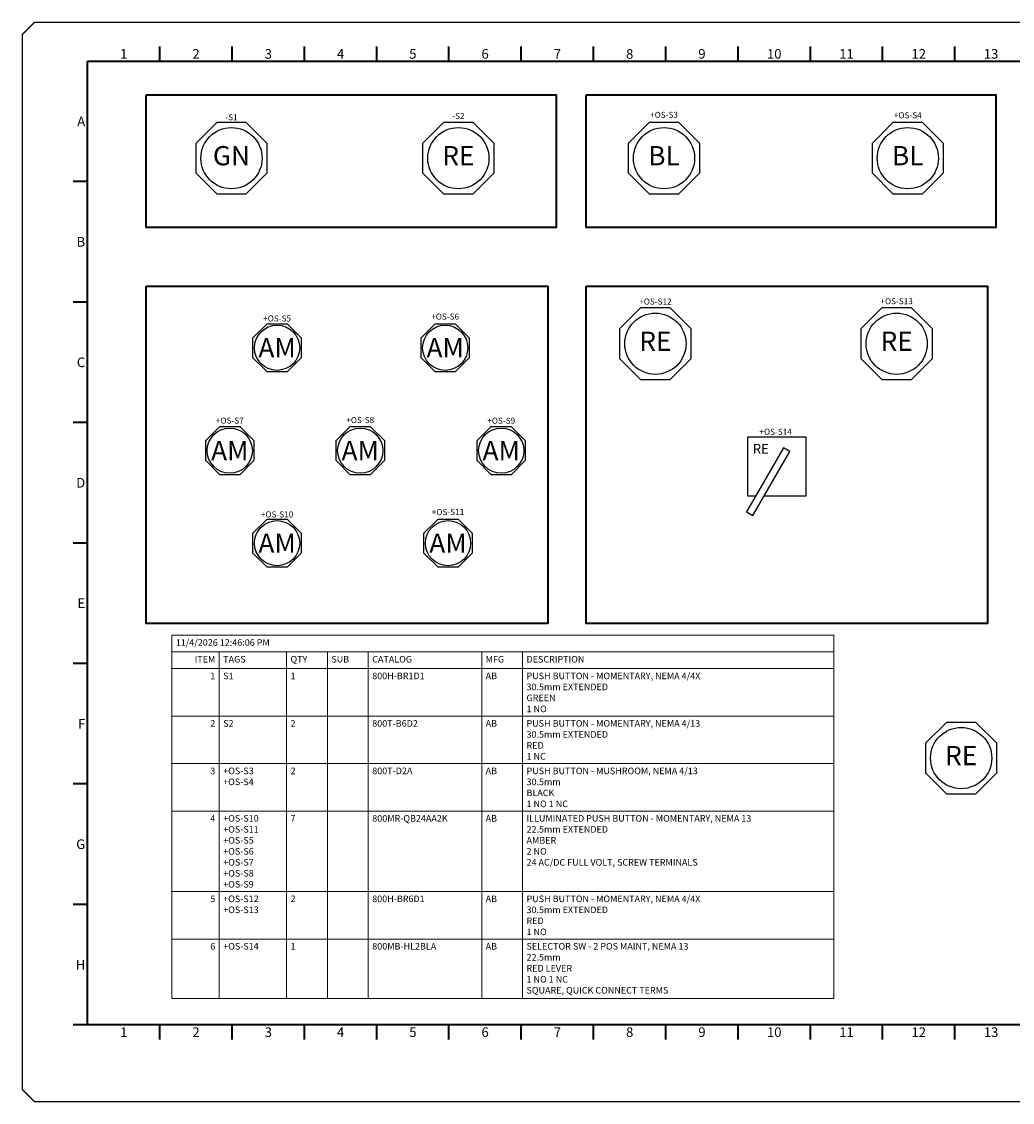
# Model space of a CAD drawing. Units: inches. Extents: x 0 to 33.5, y 0 to 22.4.
# Tile 1 of 2: x 0 to 20.6, y 0 to 22.4. Entities that reach past the tile are written whole.
import ezdxf
from ezdxf.enums import TextEntityAlignment as Align

# ---------------------------------------------------------------- set-up
doc = ezdxf.new("R2010")
doc.units = ezdxf.units.IN
doc.header["$MEASUREMENT"] = 0
for name, color, linetype, lineweight in [('E-ANNO-TABL', 3, 'Continuous', 18), ('E-ANNO-TTLB', 7, 'Continuous', 35), ('E-EQPM-PNLS', 4, 'Continuous', 35), ('PSYMS', 7, 'Continuous', 25)]:
    doc.layers.add(name, color=color, linetype=linetype, lineweight=lineweight)
for name, color, linetype in [('PMISC', 7, 'Continuous'), ('PTAG', 150, 'Continuous'), ('TITLE', 7, 'Continuous')]:
    doc.layers.add(name, color=color, linetype=linetype)
doc.styles.add('ITALIC', font='ITALIC')
doc.styles.add('SIMPLEX', font='SIMPLEX')
doc.styles.add('WD', font='romans.shx')

# ---------------------------------------------------------------- blocks, each defined once
blk = doc.blocks.new('NO_NUM_acade_title')
at = {"layer": 'TITLE', "const_width": 0.0312}
blk.add_lwpolyline([(30.594, 0.281), (30.594, 22.177), (30.344, 22.427), (0.281, 22.427), (0.031, 22.177), (0.031, 0.281), (0.281, 0.031), (30.344, 0.031)], close=True, dxfattribs=at)
at = {"layer": 'TITLE', "style": 'ITALIC'}
for tag, height, p in [('TITLE#1', 0.125, (32.156, 3.406)), ('TITLE#2', 0.125, (32.156, 3.204)), ('TITLE#3', 0.125, (32.156, 3.001)), ('TITLE#4', 0.125, (32.156, 2.799)), ('DWG#', 0.2, (32.156, 0.826))]:
    blk.add_attdef(tag, text='', height=height, dxfattribs=at).set_placement(p, align=Align.CENTER)
at = {"layer": 'TITLE', "style": 'SIMPLEX'}
blk.add_attdef('CAD#', (30.826, 1.958), '', height=0.0938, rotation=90, dxfattribs=at)
at = {"layer": 'TITLE'}
for tag, p, height, style in [('JOB#', (31.464, 1.644), 0.0938, 'SIMPLEX'), ('SCALE', (31.353, 1.344), 0.0938, 'SIMPLEX'), ('DATE', (32.408, 1.344), 0.0938, 'SIMPLEX'), ('SHTS', (32.532, 0.25), 0.2, 'ITALIC')]:
    blk.add_attdef(tag, p, '', height=height, dxfattribs=dict(at, style=style))
at = {"layer": 'TITLE', "style": 'ITALIC'}
blk.add_attdef('SH#', text='', height=0.2, dxfattribs=at).set_placement((31.881, 0.25), align=Align.RIGHT)
at = {"layer": 'TITLE', "flags": 9}
blk.add_attdef('WD_TB', (31.219, 0.031), '', height=0.125, dxfattribs=at)
blk = doc.blocks.new('ABPB3G')
for p, q in [((-0.307, 0.742), (-0.742, 0.307)), ((0.307, 0.742), (-0.307, 0.742)), ((0.742, 0.307), (0.307, 0.742)), ((-0.742, 0.307), (-0.742, -0.307)), ((0.742, -0.307), (0.742, 0.307)), ((-0.742, -0.307), (-0.307, -0.742)), ((0.307, -0.742), (0.742, -0.307)), ((-0.307, -0.742), (0.307, -0.742))]:
    blk.add_line(p, q)
blk.add_circle((0, 0), 0.635)
at = {"style": 'WD'}
blk.add_attdef('COLOR', text='', height=0.4, dxfattribs=at).set_placement((0, 0), align=Align.MIDDLE)
blk = doc.blocks.new('ABPB3R')
for p, q in [((-0.307, 0.742), (-0.742, 0.307)), ((0.307, 0.742), (-0.307, 0.742)), ((0.742, 0.307), (0.307, 0.742)), ((-0.742, 0.307), (-0.742, -0.307)), ((0.742, -0.307), (0.742, 0.307)), ((-0.742, -0.307), (-0.307, -0.742)), ((0.307, -0.742), (0.742, -0.307)), ((-0.307, -0.742), (0.307, -0.742))]:
    blk.add_line(p, q)
blk.add_circle((0, 0), 0.635)
at = {"style": 'WD'}
blk.add_attdef('COLOR', text='', height=0.4, dxfattribs=at).set_placement((0, 0), align=Align.MIDDLE)
blk = doc.blocks.new('ABPB3B')
for p, q in [((-0.307, 0.742), (-0.742, 0.307)), ((0.307, 0.742), (-0.307, 0.742)), ((0.742, 0.307), (0.307, 0.742)), ((-0.742, 0.307), (-0.742, -0.307)), ((0.742, -0.307), (0.742, 0.307)), ((-0.742, -0.307), (-0.307, -0.742)), ((0.307, -0.742), (0.742, -0.307)), ((-0.307, -0.742), (0.307, -0.742))]:
    blk.add_line(p, q)
blk.add_circle((0, 0), 0.635)
at = {"style": 'WD'}
blk.add_attdef('COLOR', text='', height=0.4, dxfattribs=at).set_placement((0, 0), align=Align.MIDDLE)
blk = doc.blocks.new('ABPB2A')
for p, q in [((-0.5, 0.207), (-0.207, 0.5)), ((-0.207, 0.5), (0.207, 0.5)), ((0.207, 0.5), (0.5, 0.207)), ((-0.5, -0.207), (-0.5, 0.207)), ((0.5, 0.207), (0.5, -0.207)), ((-0.207, -0.5), (-0.5, -0.207)), ((0.5, -0.207), (0.207, -0.5)), ((0.207, -0.5), (-0.207, -0.5))]:
    blk.add_line(p, q)
blk.add_circle((0, 0), 0.469)
at = {"style": 'WD'}
blk.add_attdef('COLOR', text='', height=0.4, dxfattribs=at).set_placement((0, 0), align=Align.MIDDLE_CENTER)
blk = doc.blocks.new('ABSS2QLMR')
for p, q in [((-0.609, 0.609), (-0.609, -0.609)), ((0.609, 0.609), (-0.609, 0.609)), ((0.609, -0.609), (0.609, 0.609)), ((0.138, 0.389), (-0.627, -0.937)), ((-0.498, -1.012), (0.268, 0.314)), ((0.268, 0.314), (0.138, 0.389)), ((-0.609, -0.609), (-0.438, -0.609)), ((-0.265, -0.609), (0.609, -0.609)), ((-0.627, -0.937), (-0.498, -1.012))]:
    blk.add_line(p, q)
at = {"style": 'WD'}
blk.add_attdef('COLOR', text='', height=0.2, dxfattribs=at).set_placement((-0.498, 0.371), align=Align.MIDDLE_LEFT)
blk = doc.blocks.new('*T12')
at = {"layer": 'E-ANNO-TABL', "transparency": 16777216}
for p, q in [((0, 0), (13.74, 0)), ((0, 0), (0, -7.54)), ((13.74, 0), (13.74, -7.54)), ((0, -0.347), (13.74, -0.347)), ((0.985, -0.347), (0.985, -7.54)), ((2.381, -0.347), (2.381, -7.54)), ((3.23, -0.347), (3.23, -7.54)), ((4.078, -0.347), (4.078, -7.54)), ((6.432, -0.347), (6.432, -7.54)), ((7.28, -0.347), (7.28, -7.54)), ((0, -0.693), (13.74, -0.693)), ((0, -1.679), (13.74, -1.679)), ((0, -2.664), (13.74, -2.664)), ((0, -3.649), (13.74, -3.649)), ((0, -5.319), (13.74, -5.319)), ((0, -6.304), (13.74, -6.304)), ((0, -7.54), (13.74, -7.54))]:
    blk.add_line(p, q, dxfattribs=at)
at = {"layer": 'E-ANNO-TABL', "color": 0, "transparency": 16777216}
for s, insert, char_height, width, attachment_point in [('11/4/2026 12:46:06 PM', (0.082, -0.082), 0.13685, 13.57538, 1), ('ITEM', (0.903, -0.429), 0.1368, 0.82109, 3), ('TAGS', (1.067, -0.429), 0.1368, 1.23164, 1), ('QTY', (2.463, -0.429), 0.1368, 0.68424, 1), ('SUB', (3.312, -0.429), 0.1368, 0.68424, 1), ('CATALOG', (4.16, -0.429), 0.1368, 2.18958, 1), ('MFG', (6.514, -0.429), 0.1368, 0.68424, 1), ('DESCRIPTION', (7.362, -0.429), 0.13685, 6.29504, 1), ('1\\P\\P\\P', (0.903, -0.775), 0.137, 0.82109, 3), ('S1\\P\\P\\P', (1.067, -0.775), 0.1368, 1.23164, 1), ('1\\P\\P\\P', (2.463, -0.775), 0.137, 0.68424, 1), ('\\P\\P\\P', (3.312, -0.775), 0.137, 0.68424, 1), ('800H-BR1D1\\P\\P\\P', (4.16, -0.775), 0.1368, 2.18958, 1), ('AB\\P\\P\\P', (6.514, -0.775), 0.1368, 0.68424, 1), ('PUSH BUTTON - MOMENTARY, NEMA 4/4X\\P30.5mm EXTENDED\\PGREEN\\P1 NO', (7.362, -0.775), 0.13685, 6.29504, 1), ('2\\P\\P\\P', (0.903, -1.761), 0.137, 0.82109, 3), ('S2\\P\\P\\P', (1.067, -1.761), 0.1368, 1.23164, 1), ('2\\P\\P\\P', (2.463, -1.761), 0.137, 0.68424, 1), ('\\P\\P\\P', (3.312, -1.761), 0.137, 0.68424, 1), ('800T-B6D2\\P\\P\\P', (4.16, -1.761), 0.1368, 2.18958, 1), ('AB\\P\\P\\P', (6.514, -1.761), 0.1368, 0.68424, 1), ('PUSH BUTTON - MOMENTARY, NEMA 4/13\\P30.5mm EXTENDED\\PRED\\P1 NC', (7.362, -1.761), 0.13685, 6.29504, 1), ('3\\P\\P\\P', (0.903, -2.746), 0.137, 0.82109, 3), ('+OS-S3\\P+OS-S4\\P\\P', (1.067, -2.746), 0.1368, 1.23164, 1), ('2\\P\\P\\P', (2.463, -2.746), 0.137, 0.68424, 1), ('\\P\\P\\P', (3.312, -2.746), 0.137, 0.68424, 1), ('800T-D2A\\P\\P\\P', (4.16, -2.746), 0.1368, 2.18958, 1), ('AB\\P\\P\\P', (6.514, -2.746), 0.1368, 0.68424, 1), ('PUSH BUTTON - MUSHROOM, NEMA 4/13\\P30.5mm\\PBLACK\\P1 NO 1 NC', (7.362, -2.746), 0.13685, 6.29504, 1), ('4\\P\\P\\P\\P\\P\\P', (0.903, -3.731), 0.137, 0.82109, 3), ('+OS-S10\\P+OS-S11\\P+OS-S5\\P+OS-S6\\P+OS-S7\\P+OS-S8\\P+OS-S9', (1.067, -3.731), 0.1368, 1.23164, 1), ('7\\P\\P\\P\\P\\P\\P', (2.463, -3.731), 0.137, 0.68424, 1), ('\\P\\P\\P\\P\\P\\P', (3.312, -3.731), 0.137, 0.68424, 1), ('800MR-QB24AA2K\\P\\P\\P\\P\\P\\P', (4.16, -3.731), 0.13685, 2.18958, 1), ('AB\\P\\P\\P\\P\\P\\P', (6.514, -3.731), 0.1368, 0.68424, 1), ('ILLUMINATED PUSH BUTTON - MOMENTARY, NEMA 13\\P22.5mm EXTENDED\\PAMBER\\P2 NO\\P24 AC/DC FULL VOLT, SCREW TERMINALS\\P\\P', (7.362, -3.731), 0.13685, 6.29504, 1), ('5\\P\\P\\P', (0.903, -5.401), 0.137, 0.82109, 3), ('+OS-S12\\P+OS-S13\\P\\P', (1.067, -5.401), 0.1368, 1.23164, 1), ('2\\P\\P\\P', (2.463, -5.401), 0.137, 0.68424, 1), ('\\P\\P\\P', (3.312, -5.401), 0.137, 0.68424, 1), ('800H-BR6D1\\P\\P\\P', (4.16, -5.401), 0.1368, 2.18958, 1), ('AB\\P\\P\\P', (6.514, -5.401), 0.1368, 0.68424, 1), ('PUSH BUTTON - MOMENTARY, NEMA 4/4X\\P30.5mm EXTENDED\\PRED\\P1 NO', (7.362, -5.401), 0.13685, 6.29504, 1), ('6\\P\\P\\P\\P', (0.903, -6.386), 0.137, 0.82109, 3), ('+OS-S14\\P\\P\\P\\P', (1.067, -6.386), 0.1368, 1.23164, 1), ('1\\P\\P\\P\\P', (2.463, -6.386), 0.137, 0.68424, 1), ('\\P\\P\\P\\P', (3.312, -6.386), 0.137, 0.68424, 1), ('800MB-HL2BLA\\P\\P\\P\\P', (4.16, -6.386), 0.13685, 2.18958, 1), ('AB\\P\\P\\P\\P', (6.514, -6.386), 0.1368, 0.68424, 1), ('SELECTOR SW - 2 POS MAINT, NEMA 13\\P22.5mm\\PRED LEVER\\P1 NO 1 NC\\PSQUARE, QUICK CONNECT TERMS', (7.362, -6.386), 0.13685, 6.29504, 1)]:
    blk.add_mtext(s, dxfattribs=dict(at, insert=insert, char_height=char_height, width=width, attachment_point=attachment_point))

msp = doc.modelspace()

# ---------------------------------------------------------------- linework, layer by layer
at = {"layer": 'E-ANNO-TTLB'}
for p, q in [((2.886, 21.623), (2.886, 21.923)), ((4.386, 21.623), (4.386, 21.923)), ((5.886, 21.623), (5.886, 21.923)), ((7.386, 21.623), (7.386, 21.923)), ((8.886, 21.623), (8.886, 21.923)), ((10.386, 21.623), (10.386, 21.923)), ((11.886, 21.623), (11.886, 21.923)), ((13.386, 21.623), (13.386, 21.923)), ((14.886, 21.623), (14.886, 21.923)), ((16.386, 21.623), (16.386, 21.923)), ((17.886, 21.623), (17.886, 21.923)), ((19.386, 21.623), (19.386, 21.923)), ((1.386, 19.123), (1.086, 19.123)), ((1.386, 16.623), (1.086, 16.623)), ((1.386, 14.123), (1.086, 14.123)), ((1.386, 11.623), (1.086, 11.623)), ((1.386, 9.123), (1.086, 9.123)), ((1.386, 6.623), (1.086, 6.623)), ((1.386, 4.123), (1.086, 4.123)), ((1.386, 1.623), (1.086, 1.623)), ((2.886, 1.323), (2.886, 1.623)), ((4.386, 1.323), (4.386, 1.623)), ((5.886, 1.323), (5.886, 1.623)), ((7.386, 1.323), (7.386, 1.623)), ((8.886, 1.323), (8.886, 1.623)), ((10.386, 1.323), (10.386, 1.623)), ((11.886, 1.323), (11.886, 1.623)), ((13.386, 1.323), (13.386, 1.623)), ((14.886, 1.323), (14.886, 1.623)), ((16.386, 1.323), (16.386, 1.623)), ((17.886, 1.323), (17.886, 1.623)), ((19.386, 1.323), (19.386, 1.623))]:
    msp.add_line(p, q, dxfattribs=at)
msp.add_lwpolyline([(1.386, 21.623), (25.386, 21.623), (25.386, 1.623), (1.386, 1.623)], close=True, dxfattribs=at)
at = {"layer": 'E-EQPM-PNLS'}
for points in [[(2.602, 20.924), (11.107, 20.924), (11.107, 18.17), (2.602, 18.17)], [(11.731, 20.924), (20.236, 20.924), (20.236, 18.17), (11.731, 18.17)], [(2.602, 16.953), (10.936, 16.953), (10.936, 9.95), (2.602, 9.95)], [(11.731, 16.953), (20.065, 16.953), (20.065, 9.95), (11.731, 9.95)]]:
    msp.add_lwpolyline(points, close=True, dxfattribs=at)

# ---------------------------------------------------------------- block references
msp.add_blockref('*T12', (3.133, 9.709))
at = {"layer": 'E-ANNO-TTLB'}
msp.add_blockref('NO_NUM_acade_title', (0, 0), dxfattribs=at)
at = {"layer": 'PSYMS'}
ref = msp.add_blockref('ABPB3G', (4.371, 19.609), dxfattribs=at)
ref.add_attrib('COLOR', 'GN', dxfattribs={"layer": 'PMISC', "height": 0.4, "style": 'WD'}).set_placement((4.371, 19.609), align=Align.MIDDLE)
ref.add_attrib('P_TAG1', '-S1', dxfattribs={"layer": 'PTAG', "height": 0.125, "style": 'WD', "flags": 8}).set_placement((4.371, 20.459), align=Align.MIDDLE_CENTER)
ref = msp.add_blockref('ABPB3R', (9.081, 19.609), dxfattribs=at)
ref.add_attrib('COLOR', 'RE', dxfattribs={"layer": 'PMISC', "height": 0.4, "style": 'WD'}).set_placement((9.081, 19.609), align=Align.MIDDLE)
ref.add_attrib('P_TAG1', '-S2', dxfattribs={"layer": 'PTAG', "height": 0.125, "style": 'WD', "flags": 8}).set_placement((9.081, 20.484), align=Align.MIDDLE_CENTER)
ref = msp.add_blockref('ABPB3B', (13.349, 19.609), dxfattribs=at)
ref.add_attrib('COLOR', 'BL', dxfattribs={"layer": 'PMISC', "height": 0.4, "style": 'WD'}).set_placement((13.349, 19.609), align=Align.MIDDLE)
ref.add_attrib('P_TAG1', '+OS-S3', dxfattribs={"layer": 'PTAG', "height": 0.125, "style": 'WD', "flags": 8}).set_placement((13.349, 20.508), align=Align.MIDDLE_CENTER)
ref = msp.add_blockref('ABPB3B', (18.408, 19.609), dxfattribs=at)
ref.add_attrib('COLOR', 'BL', dxfattribs={"layer": 'PMISC', "height": 0.4, "style": 'WD'}).set_placement((18.408, 19.609), align=Align.MIDDLE)
ref.add_attrib('P_TAG1', '+OS-S4', dxfattribs={"layer": 'PTAG', "height": 0.125, "style": 'WD', "flags": 8}).set_placement((18.408, 20.5), align=Align.MIDDLE_CENTER)
ref = msp.add_blockref('ABPB3R', (13.17, 15.758), dxfattribs=at)
ref.add_attrib('COLOR', 'RE', dxfattribs={"layer": 'PMISC', "height": 0.4, "style": 'WD'}).set_placement((13.17, 15.758), align=Align.MIDDLE)
ref.add_attrib('P_TAG1', '+OS-S12', dxfattribs={"layer": 'PTAG', "height": 0.125, "style": 'WD', "flags": 8}).set_placement((13.17, 16.634), align=Align.MIDDLE_CENTER)
ref = msp.add_blockref('ABPB3R', (18.177, 15.758), dxfattribs=at)
ref.add_attrib('COLOR', 'RE', dxfattribs={"layer": 'PMISC', "height": 0.4, "style": 'WD'}).set_placement((18.177, 15.758), align=Align.MIDDLE)
ref.add_attrib('P_TAG1', '+OS-S13', dxfattribs={"layer": 'PTAG', "height": 0.125, "style": 'WD', "flags": 8}).set_placement((18.177, 16.641), align=Align.MIDDLE_CENTER)
ref = msp.add_blockref('ABPB2A', (8.807, 15.674), dxfattribs=at)
ref.add_attrib('COLOR', 'AM', dxfattribs={"layer": 'PMISC', "height": 0.4, "style": 'WD'}).set_placement((8.807, 15.674), align=Align.MIDDLE_CENTER)
ref.add_attrib('P_TAG1', '+OS-S6', dxfattribs={"layer": 'PTAG', "height": 0.125, "style": 'WD', "flags": 8}).set_placement((8.807, 16.322), align=Align.MIDDLE_CENTER)
ref = msp.add_blockref('ABPB2A', (5.318, 15.674), dxfattribs=at)
ref.add_attrib('COLOR', 'AM', dxfattribs={"layer": 'PMISC', "height": 0.4, "style": 'WD'}).set_placement((5.318, 15.674), align=Align.MIDDLE_CENTER)
ref.add_attrib('P_TAG1', '+OS-S5', dxfattribs={"layer": 'PTAG', "height": 0.125, "style": 'WD', "flags": 8}).set_placement((5.318, 16.283), align=Align.MIDDLE_CENTER)
ref = msp.add_blockref('ABPB2A', (4.336, 13.54), dxfattribs=at)
ref.add_attrib('COLOR', 'AM', dxfattribs={"layer": 'PMISC', "height": 0.4, "style": 'WD'}).set_placement((4.336, 13.54), align=Align.MIDDLE_CENTER)
ref.add_attrib('P_TAG1', '+OS-S7', dxfattribs={"layer": 'PTAG', "height": 0.125, "style": 'WD', "flags": 8}).set_placement((4.336, 14.164), align=Align.MIDDLE_CENTER)
ref = msp.add_blockref('ABPB2A', (7.044, 13.54), dxfattribs=at)
ref.add_attrib('COLOR', 'AM', dxfattribs={"layer": 'PMISC', "height": 0.4, "style": 'WD'}).set_placement((7.044, 13.54), align=Align.MIDDLE_CENTER)
ref.add_attrib('P_TAG1', '+OS-S8', dxfattribs={"layer": 'PTAG', "height": 0.125, "style": 'WD', "flags": 8}).set_placement((7.044, 14.174), align=Align.MIDDLE_CENTER)
ref = msp.add_blockref('ABPB2A', (9.97, 13.54), dxfattribs=at)
ref.add_attrib('COLOR', 'AM', dxfattribs={"layer": 'PMISC', "height": 0.4, "style": 'WD'}).set_placement((9.97, 13.54), align=Align.MIDDLE_CENTER)
ref.add_attrib('P_TAG1', '+OS-S9', dxfattribs={"layer": 'PTAG', "height": 0.125, "style": 'WD', "flags": 8}).set_placement((9.97, 14.161), align=Align.MIDDLE_CENTER)
ref = msp.add_blockref('ABSS2QLMR', (15.69, 13.208), dxfattribs=at)
ref.add_attrib('COLOR', 'RE', dxfattribs={"layer": 'PMISC', "height": 0.2, "style": 'WD'}).set_placement((15.191, 13.578), align=Align.MIDDLE_LEFT)
ref.add_attrib('P_TAG1', '+OS-S14', dxfattribs={"layer": 'PTAG', "height": 0.125, "style": 'WD', "flags": 8}).set_placement((15.665, 13.931), align=Align.MIDDLE_CENTER)
ref = msp.add_blockref('ABPB2A', (5.318, 11.62), dxfattribs=at)
ref.add_attrib('COLOR', 'AM', dxfattribs={"layer": 'PMISC', "height": 0.4, "style": 'WD'}).set_placement((5.318, 11.62), align=Align.MIDDLE_CENTER)
ref.add_attrib('P_TAG1', '+OS-S10', dxfattribs={"layer": 'PTAG', "height": 0.125, "style": 'WD', "flags": 8}).set_placement((5.318, 12.216), align=Align.MIDDLE_CENTER)
ref = msp.add_blockref('ABPB2A', (8.866, 11.62), dxfattribs=at)
ref.add_attrib('COLOR', 'AM', dxfattribs={"layer": 'PMISC', "height": 0.4, "style": 'WD'}).set_placement((8.866, 11.62), align=Align.MIDDLE_CENTER)
ref.add_attrib('P_TAG1', '+OS-S11', dxfattribs={"layer": 'PTAG', "height": 0.125, "style": 'WD', "flags": 8}).set_placement((8.866, 12.265), align=Align.MIDDLE_CENTER)
ref = msp.add_blockref('ABPB3R', (19.516, 7.16), dxfattribs=at)
ref.add_attrib('COLOR', 'RE', dxfattribs={"layer": 'PMISC', "height": 0.4, "style": 'WD'}).set_placement((19.516, 7.16), align=Align.MIDDLE)

# ---------------------------------------------------------------- texts
at = {"layer": 'E-ANNO-TTLB'}
for s, p in [('1', (2.136, 21.673)), ('2', (3.636, 21.673)), ('3', (5.136, 21.673)), ('4', (6.636, 21.673)), ('5', (8.136, 21.673)), ('6', (9.636, 21.673)), ('7', (11.136, 21.673)), ('8', (12.636, 21.673)), ('9', (14.136, 21.673)), ('10', (15.636, 21.673)), ('11', (17.136, 21.673)), ('12', (18.636, 21.673)), ('13', (20.136, 21.673)), ('1', (2.136, 1.373)), ('2', (3.636, 1.373)), ('3', (5.136, 1.373)), ('4', (6.636, 1.373)), ('5', (8.136, 1.373)), ('6', (9.636, 1.373)), ('7', (11.136, 1.373)), ('8', (12.636, 1.373)), ('9', (14.136, 1.373)), ('10', (15.636, 1.373)), ('11', (17.136, 1.373)), ('12', (18.636, 1.373)), ('13', (20.136, 1.373))]:
    msp.add_text(s, height=0.2, dxfattribs=at).set_placement(p, align=Align.CENTER)
for s, p in [('A', (1.336, 20.373)), ('B', (1.336, 17.873)), ('C', (1.336, 15.373)), ('D', (1.336, 12.873)), ('E', (1.336, 10.373)), ('F', (1.336, 7.873)), ('G', (1.336, 5.373)), ('H', (1.336, 2.873))]:
    msp.add_text(s, height=0.2, dxfattribs=at).set_placement(p, align=Align.MIDDLE_RIGHT)

doc.saveas('drawing.dxf')
